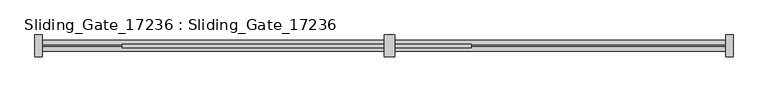
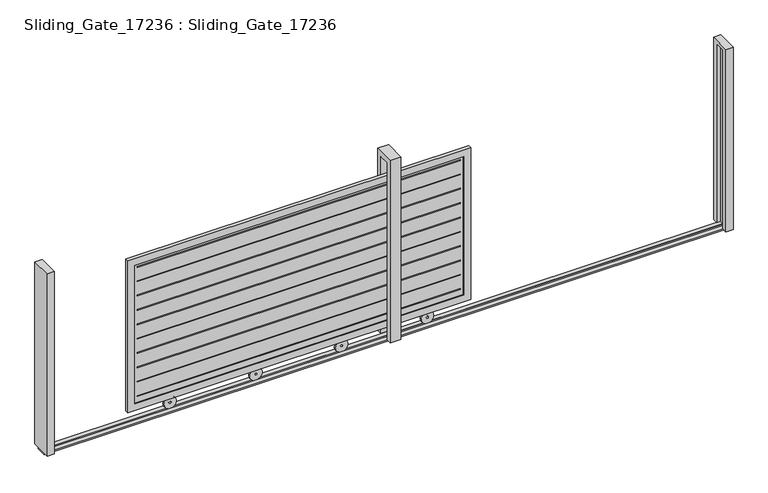
"""IFC4 building model written with IfcOpenShell, lengths in millimetres: geographic element geometry, Sliding_Gate_17236 : Sliding_Gate_17236."""

from ifc_helpers import new_model, si_unit, point, frame, frame_2d, origin, place, context, project, spatial, polyline, circle_curve, trimmed, segment, composite_curve, outline, extrude, faceted_brep, source, transform, mapped, element, save


def sliding_gate_17236_sliding_gate_17236_fdb57db6(model_context):
    return source(origin(), model_context, "Body", "SolidModel", [
        faceted_brep([(4826.0, 152.4, 0.0), (4876.8, 152.4, 0.0), (4876.8, 0.0, 0.0), (4826.0, 0.0, 0.0), (4826.0, 38.1, 0.0), (4851.4, 38.1, 0.0), (4851.4, 114.3, 0.0), (4826.0, 114.3, 0.0), (4851.4, 114.3, 1346.2), (4826.0, 114.3, 1346.2), (4851.4, 38.1, 1346.2), (4826.0, 38.1, 1346.2), (4826.0, 0.0, 1371.6), (4876.8, 0.0, 1371.6), (4876.8, 152.4, 1371.6), (4826.0, 152.4, 1371.6)], [[[0, 1, 2, 3, 4, 5, 6, 7]], [[6, 8, 9, 7]], [[5, 10, 8, 6]], [[4, 11, 10, 5]], [[12, 3, 2, 13]], [[13, 2, 1, 14]], [[14, 1, 0, 15]], [[11, 4, 3, 12, 15, 0, 7, 9]], [[9, 8, 10, 11]], [[12, 13, 14, 15]]]),
        extrude(outline(composite_curve([segment(trimmed(circle_curve(frame_2d((43.1280612, 914.4)), 44.45), [point((43.1280612, 869.95))], [point((43.1280612, 958.85))], False, "CARTESIAN"), True, "CONTINUOUS"), segment(trimmed(circle_curve(frame_2d((43.1280612, 914.4)), 44.45), [point((43.1280612, 958.85))], [point((43.1280612, 869.95))], False, "CARTESIAN"), True, "CONTINUOUS")], self_intersect=False), holes=[composite_curve([segment(trimmed(circle_curve(frame_2d((43.1280612, 914.4)), 6.35), [point((43.1280612, 908.05))], [point((43.1280612, 920.75))], True, "CARTESIAN"), True, "CONTINUOUS"), segment(trimmed(circle_curve(frame_2d((43.1280612, 914.4)), 6.35), [point((43.1280612, 920.75))], [point((43.1280612, 908.05))], True, "CARTESIAN"), True, "CONTINUOUS")], self_intersect=False)]), frame((0.0, 69.85, 0.0), z_axis=(0.0, 1.0, 0.0), x_axis=(0.0, 0.0, 1.0)), (0.0, 0.0, 1.0), 12.7),
        extrude(outline(composite_curve([segment(trimmed(circle_curve(frame_2d((43.1280612, 2133.6)), 44.45), [point((43.1280612, 2089.15))], [point((43.1280612, 2178.05))], False, "CARTESIAN"), True, "CONTINUOUS"), segment(trimmed(circle_curve(frame_2d((43.1280612, 2133.6)), 44.45), [point((43.1280612, 2178.05))], [point((43.1280612, 2089.15))], False, "CARTESIAN"), True, "CONTINUOUS")], self_intersect=False), holes=[composite_curve([segment(trimmed(circle_curve(frame_2d((43.1280612, 2133.6)), 6.35), [point((43.1280612, 2127.25))], [point((43.1280612, 2139.95))], True, "CARTESIAN"), True, "CONTINUOUS"), segment(trimmed(circle_curve(frame_2d((43.1280612, 2133.6)), 6.35), [point((43.1280612, 2139.95))], [point((43.1280612, 2127.25))], True, "CARTESIAN"), True, "CONTINUOUS")], self_intersect=False)]), frame((0.0, 69.85, 0.0), z_axis=(0.0, 1.0, 0.0), x_axis=(0.0, 0.0, 1.0)), (0.0, 0.0, 1.0), 12.7),
        extrude(outline(composite_curve([segment(trimmed(circle_curve(frame_2d((43.1280612, 2743.2)), 44.45), [point((43.1280612, 2698.75))], [point((43.1280612, 2787.65))], False, "CARTESIAN"), True, "CONTINUOUS"), segment(trimmed(circle_curve(frame_2d((43.1280612, 2743.2)), 44.45), [point((43.1280612, 2787.65))], [point((43.1280612, 2698.75))], False, "CARTESIAN"), True, "CONTINUOUS")], self_intersect=False), holes=[composite_curve([segment(trimmed(circle_curve(frame_2d((43.1280612, 2743.2)), 6.35), [point((43.1280612, 2736.85))], [point((43.1280612, 2749.55))], True, "CARTESIAN"), True, "CONTINUOUS"), segment(trimmed(circle_curve(frame_2d((43.1280612, 2743.2)), 6.35), [point((43.1280612, 2749.55))], [point((43.1280612, 2736.85))], True, "CARTESIAN"), True, "CONTINUOUS")], self_intersect=False)]), frame((0.0, 69.85, 0.0), z_axis=(0.0, 1.0, 0.0), x_axis=(0.0, 0.0, 1.0)), (0.0, 0.0, 1.0), 12.7),
        extrude(outline(composite_curve([segment(trimmed(circle_curve(frame_2d((43.1280612, 1524.0)), 44.45), [point((43.1280612, 1479.55))], [point((43.1280612, 1568.45))], False, "CARTESIAN"), True, "CONTINUOUS"), segment(trimmed(circle_curve(frame_2d((43.1280612, 1524.0)), 44.45), [point((43.1280612, 1568.45))], [point((43.1280612, 1479.55))], False, "CARTESIAN"), True, "CONTINUOUS")], self_intersect=False), holes=[composite_curve([segment(trimmed(circle_curve(frame_2d((43.1280612, 1524.0)), 6.35), [point((43.1280612, 1517.65))], [point((43.1280612, 1530.35))], True, "CARTESIAN"), True, "CONTINUOUS"), segment(trimmed(circle_curve(frame_2d((43.1280612, 1524.0)), 6.35), [point((43.1280612, 1530.35))], [point((43.1280612, 1517.65))], True, "CARTESIAN"), True, "CONTINUOUS")], self_intersect=False)]), frame((0.0, 69.85, 0.0), z_axis=(0.0, 1.0, 0.0), x_axis=(0.0, 0.0, 1.0)), (0.0, 0.0, 1.0), 12.7),
        extrude(outline(polyline([(1217.8780612, 3048.0), (1217.8780612, 609.6), (74.8780612, 609.6), (74.8780612, 3048.0), (1217.8780612, 3048.0)]), holes=[polyline([(1167.0780612, 660.4), (1167.0780612, 2997.2), (125.6780612, 2997.2), (125.6780612, 660.4), (1167.0780612, 660.4)])]), frame((0.0, 63.5, 0.0), z_axis=(0.0, 1.0, 0.0), x_axis=(0.0, 0.0, 1.0)), (0.0, 0.0, 1.0), 25.4),
        extrude(outline(polyline([(1173.4280612, 3003.55), (1173.4280612, 654.05), (119.3280612, 654.05), (119.3280612, 3003.55), (1173.4280612, 3003.55)]), holes=[polyline([(1148.0280612, 679.45), (1148.0280612, 2978.15), (1141.6780612, 2978.15), (1141.6780612, 679.45), (1148.0280612, 679.45)]), polyline([(1040.0780612, 679.45), (1040.0780612, 2978.15), (1033.7280612, 2978.15), (1033.7280612, 679.45), (1040.0780612, 679.45)]), polyline([(932.1280612, 679.45), (932.1280612, 2978.15), (925.7780612, 2978.15), (925.7780612, 679.45), (932.1280612, 679.45)]), polyline([(824.1780612, 679.45), (824.1780612, 2978.15), (817.8280612, 2978.15), (817.8280612, 679.45), (824.1780612, 679.45)]), polyline([(716.2280612, 679.45), (716.2280612, 2978.15), (709.8780612, 2978.15), (709.8780612, 679.45), (716.2280612, 679.45)]), polyline([(608.2780612, 679.45), (608.2780612, 2978.15), (601.9280612, 2978.15), (601.9280612, 679.45), (608.2780612, 679.45)]), polyline([(500.3280612, 679.45), (500.3280612, 2978.15), (493.9780612, 2978.15), (493.9780612, 679.45), (500.3280612, 679.45)]), polyline([(392.3780612, 679.45), (392.3780612, 2978.15), (386.0280612, 2978.15), (386.0280612, 679.45), (392.3780612, 679.45)]), polyline([(284.4280612, 679.45), (284.4280612, 2978.15), (278.0780612, 2978.15), (278.0780612, 679.45), (284.4280612, 679.45)]), polyline([(176.4780612, 679.45), (176.4780612, 2978.15), (170.1280612, 2978.15), (170.1280612, 679.45), (176.4780612, 679.45)])]), frame((0.0, 69.85, 0.0), z_axis=(0.0, 1.0, 0.0), x_axis=(0.0, 0.0, 1.0)), (0.0, 0.0, 1.0), 12.7),
        extrude(outline(polyline([(152.4, 1371.6), (152.4, 0.0), (114.3, 0.0), (114.3, 1333.5), (38.1, 1333.5), (38.1, 0.0), (0.0, 0.0), (0.0, 1371.6), (152.4, 1371.6)])), frame((2438.4, 0.0, 0.0), z_axis=(1.0, 0.0, 0.0), x_axis=(0.0, 1.0, 0.0)), (0.0, 0.0, 1.0), 76.2),
        faceted_brep([(50.8, 152.4, 0.0), (50.8, 114.3, 0.0), (25.4, 114.3, 0.0), (25.4, 38.1, 0.0), (50.8, 38.1, 0.0), (50.8, 0.0, 0.0), (0.0, 0.0, 0.0), (0.0, 152.4, 0.0), (50.8, 114.3, 1346.2), (25.4, 114.3, 1346.2), (25.4, 38.1, 1346.2), (50.8, 38.1, 1346.2), (50.8, 0.0, 1371.6), (0.0, 0.0, 1371.6), (0.0, 152.4, 1371.6), (50.8, 152.4, 1371.6)], [[[0, 1, 2, 3, 4, 5, 6, 7]], [[2, 1, 8, 9]], [[3, 2, 9, 10]], [[4, 3, 10, 11]], [[12, 13, 6, 5]], [[13, 14, 7, 6]], [[14, 15, 0, 7]], [[11, 8, 1, 0, 15, 12, 5, 4]], [[8, 11, 10, 9]], [[12, 15, 14, 13]]]),
        extrude(outline(polyline([(83.3319524, 0.0), (114.3, 0.0), (114.3, -12.7), (38.1, -12.7), (38.1, 0.0), (68.8793004, 0.0), (68.8793004, -1.3219388), (83.3319524, -1.3219388), (83.3319524, 0.0)])), frame((0.0, 0.0, 0.0), z_axis=(1.0, 0.0, 0.0), x_axis=(0.0, 1.0, 0.0)), (0.0, 0.0, 1.0), 4876.8),
    ])


if __name__ == "__main__":
    model = new_model("IFC4")
    model_context = context("Model", 3, world=origin())
    ifc_project = project(units=[si_unit("LENGTHUNIT", "METRE", prefix="MILLI")], contexts=[model_context])
    site = spatial("IfcSite", under=ifc_project)
    building = spatial("IfcBuilding", under=site)
    placement = place(None, origin())
    sliding_gate_17236_sliding_gate_17236_shape = sliding_gate_17236_sliding_gate_17236_fdb57db6(model_context)
    element("IfcGeographicElement", 1, ObjectType="Sliding_Gate_17236 : Sliding_Gate_17236", at=placement, inside=building, context=model_context, shape_type="MappedRepresentation", body=[
        mapped(sliding_gate_17236_sliding_gate_17236_shape, transform((0.0, 0.0, 0.0), x_axis=(1.0, 0.0, 0.0), y_axis=(0.0, 1.0, 0.0), z_axis=(0.0, 0.0, 1.0))),
    ])
    save(model, "model.ifc")

# Revit data of these elements
# Type "Sliding_Gate_17236 : Sliding_Gate_17236"
#   channel width = 16' - 0"
#   Width = 8' - 0"
#   Gate open = 2' - 0"
#   stopper material = aluminium dark grey
#   panel material = wood panel
# Element 1 (IfcGeographicElement, "Sliding_Gate_17236 : Sliding_Gate_17236")
#   Materials on its faces: "wood panel", "aluminium dark grey", "black metal"
# Materials
#   "aluminium dark grey": class "Generic", colour RGB 85 85 85, transparency 0, Cost = 0
#   "wood panel": class "Generic", colour RGB 128 64 0, transparency 0, Cost = 0
#   "black metal": class "Generic", colour RGB 120 120 120, transparency 0, Cost = 0
